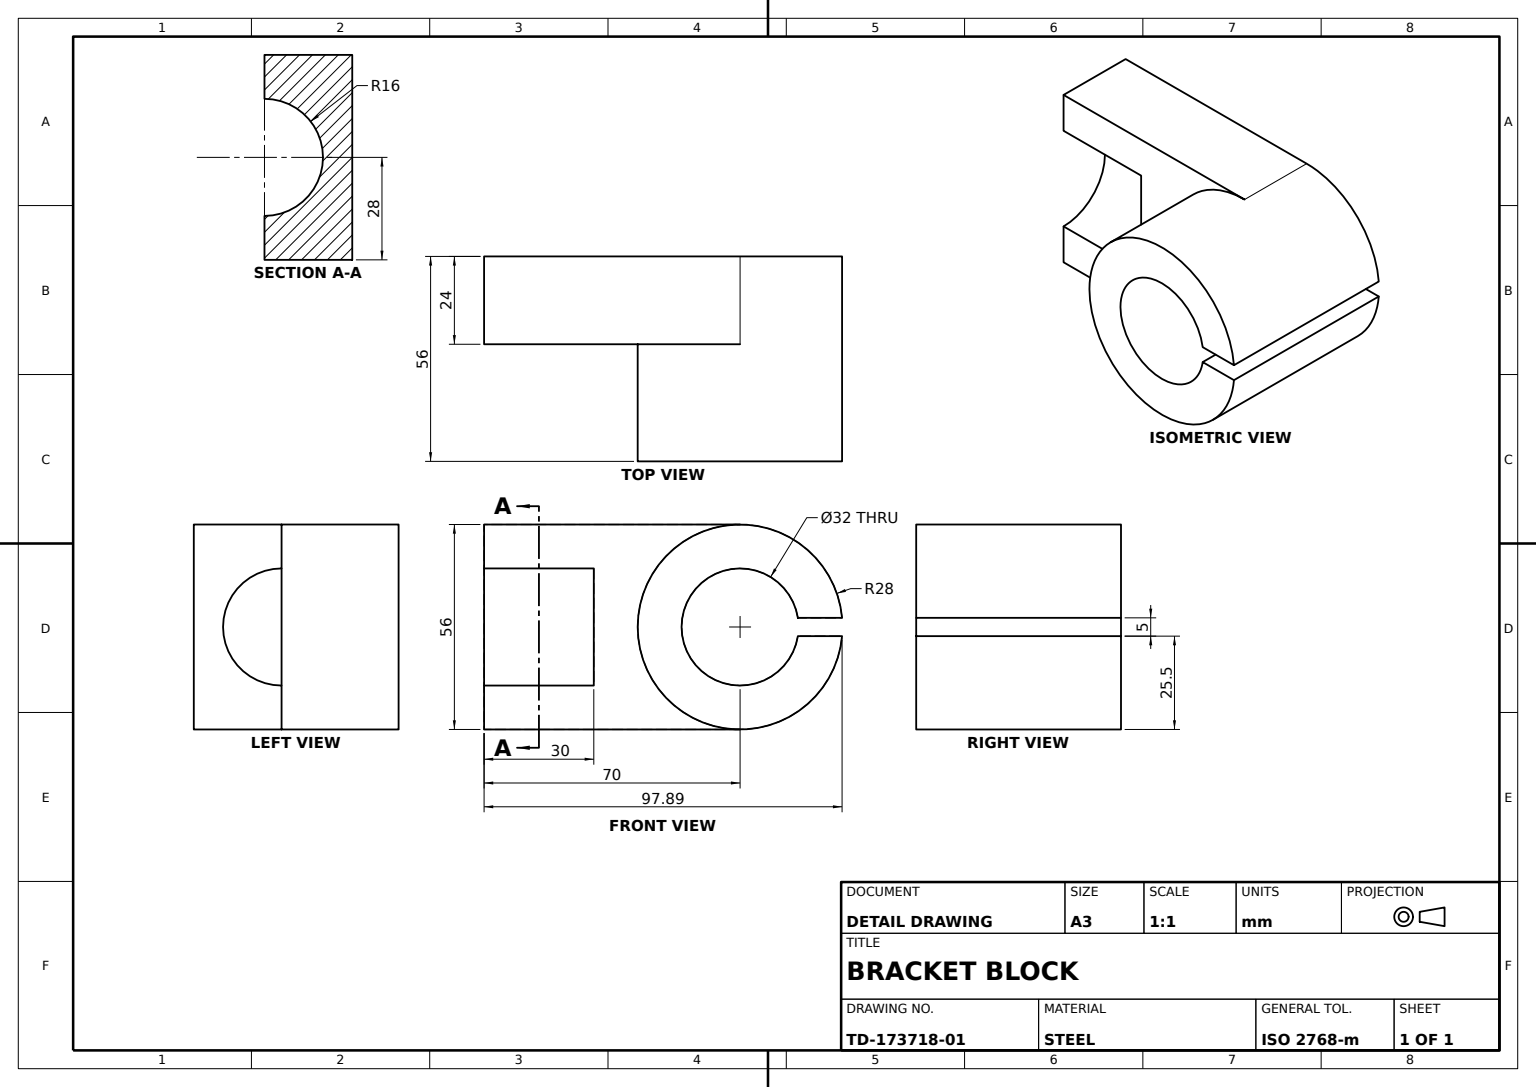
from build123d import *

# Parameters (mm, degrees)
BASE_BLOCK_SKETCH_R   = 28
BASE_BLOCK_SKETCH_R_2 = 16
BASE_BLOCK_DEPTH      = 56
CLAMP_BOSS_DEPTH      = 24
SIDE_WINDOW_CUT_DEPTH = 54
BORE_DEPTH            = 30
CLAMP_SLIT_2_5_DEPTH  = 80


with BuildPart() as part:
    # Base Block Sketch → Base Block (new body)
    with BuildSketch(Plane(origin=(0, 0, 0), x_dir=(0, 0, -1), z_dir=(1, 0, 0))):
        Circle(BASE_BLOCK_SKETCH_R)
        Circle(BASE_BLOCK_SKETCH_R_2, mode=Mode.SUBTRACT)
    extrude(amount=BASE_BLOCK_DEPTH)

    # Clamp Boss Sketch → Clamp Boss (add)
    with BuildSketch(Plane.ZY):
        Polygon((0, 0), (0, 28), (70, 28), (70, -28), (0, -28), align=None)
    extrude(amount=-CLAMP_BOSS_DEPTH)

    # Side Window Sketch → Side Window Cut (cut)
    with BuildSketch(Plane.ZY):
        with BuildLine():
            Line((0, 16), (0, -16))
            ThreePointArc((0, -16), (16, 0), (0, 16))
        make_face()
    extrude(amount=-SIDE_WINDOW_CUT_DEPTH, mode=Mode.SUBTRACT)

    # Bore Sketch → Bore (cut)
    with BuildSketch(Plane.XY.offset(70)):
        with BuildLine():
            Line((24, 16), (24, -16))
            ThreePointArc((24, -16), (8, 0), (24, 16))
        make_face()
    extrude(amount=-BORE_DEPTH, mode=Mode.SUBTRACT)

    # Clamp Slit Sketch → Clamp Slit 2.5 (cut)
    with BuildSketch(Plane(origin=(56, 0, 0), x_dir=(0, 0, -1), z_dir=(1, 0, 0))):
        Polygon((30.140731053, 0), (30.140731053, 2.5), (15.803480629, 2.5), (15.803480629, -2.5), (30.140731053, -2.5), align=None)
    extrude(amount=-CLAMP_SLIT_2_5_DEPTH, mode=Mode.SUBTRACT)


solid = part.part
